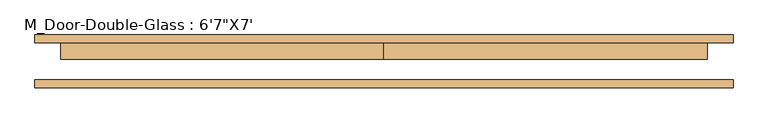
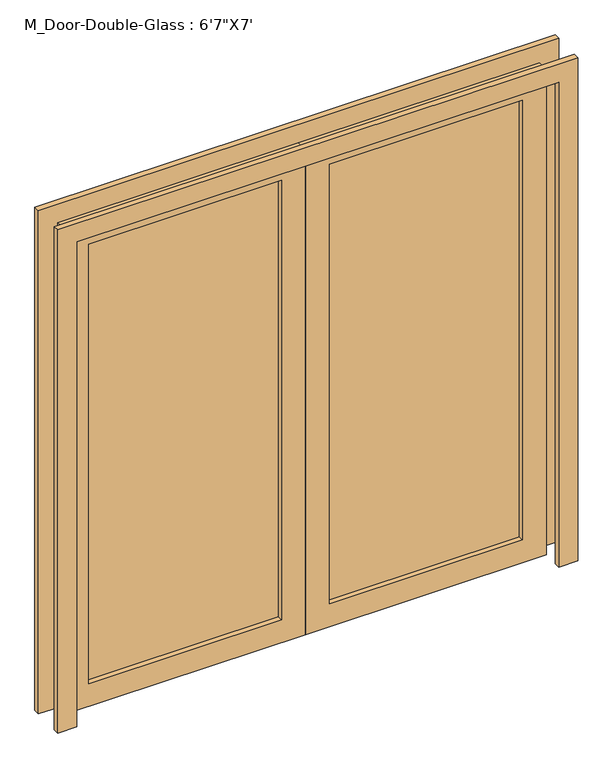
"""IFC4 building model written with IfcOpenShell, lengths in millimetres: door geometry."""

from ifc_helpers import new_model, si_unit, frame, origin, place, context, project, spatial, polyline, outline, extrude, source, transform, mapped, element, save


def door_04ab2522(model_context):
    return source(origin(), model_context, "Body", "SweptSolid", [
        extrude(outline(polyline([(2133.6, 1003.3), (2133.6, 0.0), (0.0, 0.0), (0.0, 1003.3), (2133.6, 1003.3)]), holes=[polyline([(2033.6, 903.3), (100.0, 903.3), (100.0, 100.0), (2033.6, 100.0), (2033.6, 903.3)])]), frame((0.0, 9.53125, 0.0), z_axis=(0.0, 1.0, 0.0), x_axis=(0.0, 0.0, 1.0)), (0.0, 0.0, 1.0), 50.0),
        extrude(outline(polyline([(2133.6, -1003.3), (0.0, -1003.3), (0.0, 0.0), (2133.6, 0.0), (2133.6, -1003.3)]), holes=[polyline([(2033.6, -903.3), (2033.6, -100.0), (100.0, -100.0), (100.0, -903.3), (2033.6, -903.3)])]), frame((0.0, 9.53125, 0.0), z_axis=(0.0, 1.0, 0.0), x_axis=(0.0, 0.0, 1.0)), (0.0, 0.0, 1.0), 50.0),
        extrude(outline(polyline([(-903.3, 37.70625), (-100.0, 37.70625), (-100.0, 31.35625), (-903.3, 31.35625), (-903.3, 37.70625)])), frame((0.0, 0.0, 100.0), z_axis=(0.0, 0.0, 1.0), x_axis=(1.0, 0.0, 0.0)), (0.0, 0.0, 1.0), 1933.6),
        extrude(outline(polyline([(100.0, 37.70625), (903.3, 37.70625), (903.3, 31.35625), (100.0, 31.35625), (100.0, 37.70625)])), frame((0.0, 0.0, 100.0), z_axis=(0.0, 0.0, 1.0), x_axis=(1.0, 0.0, 0.0)), (0.0, 0.0, 1.0), 1933.6),
        extrude(outline(polyline([(0.0, 1083.3), (2213.6, 1083.3), (2213.6, -1083.3), (0.0, -1083.3), (0.0, -1003.3), (2133.6, -1003.3), (2133.6, 1003.3), (0.0, 1003.3), (0.0, 1083.3)])), frame((0.0, -79.76875, 0.0), z_axis=(0.0, 1.0, 0.0), x_axis=(0.0, 0.0, 1.0)), (0.0, 0.0, 1.0), 25.0),
        extrude(outline(polyline([(0.0, 1083.3), (2213.6, 1083.3), (2213.6, -1083.3), (0.0, -1083.3), (0.0, -1003.3), (2133.6, -1003.3), (2133.6, 1003.3), (0.0, 1003.3), (0.0, 1083.3)])), frame((0.0, 59.53125, 0.0), z_axis=(0.0, 1.0, 0.0), x_axis=(0.0, 0.0, 1.0)), (0.0, 0.0, 1.0), 25.0),
    ])


if __name__ == "__main__":
    model = new_model("IFC4")
    model_context = context("Model", 3, world=origin())
    ifc_project = project(units=[si_unit("LENGTHUNIT", "METRE", prefix="MILLI")], contexts=[model_context])
    site = spatial("IfcSite", under=ifc_project)
    building = spatial("IfcBuilding", under=site)
    placement = place(None, origin())
    door_shape = door_04ab2522(model_context)
    element("IfcDoor", 1, ObjectType="M_Door-Double-Glass : 6'7\"X7'", at=placement, inside=building, context=model_context, shape_type="MappedRepresentation", body=[
        mapped(door_shape, transform((0.0, 0.0, 0.0), x_axis=(1.0, 0.0, 0.0), y_axis=(0.0, 1.0, 0.0), z_axis=(0.0, 0.0, 1.0))),
    ])
    save(model, "model.ifc")

# Revit data of these elements
# Type "M_Door-Double-Glass : 6'7\"X7'"
#   Type Mark = "16"
#   Construction Type Id = "opn-d45"
#   Assembly Code = "C1020"
#   Analytic Construction = "Wood frame, double glass door "
#   W = 3' - 3 1/2"
#   Thickness = 0' - 1.9685"
#   Thermal Resistance (R) = 1.8150 (h·ft²·°F)/BTU
#   Swing Angle [instance default] = 90.00°
#   Heat Transfer Coefficient (U) = 0.5510 BTU/(h·ft²·°F)
#   Height = 7' - 0"
#   Bottom Rail = 0' - 3.93701"
#   Top Rail = 0' - 3.93701"
#   Stiles = 0' - 3.93701"
#   Trim Projection = 0' - 0.98425"
#   Trim Width = 0' - 3.14961"
#   Width = 6' - 7"
#   Define Thermal Properties by = 1
#   Glazing = Glass
#   Panel Material = Wood - Birch - Solid Stained Light Low Gloss
#   Trim Material = Paint - Sienna
#   Visual Light Transmittance = 0
#   Solar Heat Gain Coefficient = 0
#   Function = (empty or 0)
#   Wall Closure = (empty or 0)
# Element 1 (IfcDoor, "M_Door-Double-Glass : 6'7\"X7'")
#   Materials on its faces: "Wood - Birch - Solid Stained Light Low Gloss", "Paint - Sienna", "Glass"
# Materials
#   "Glass": class "Glass", colour RGB 0 128 192, transparency 0.75, Description = "Soda Lime Glass", Cost = 0
#   "Wood - Birch - Solid Stained Light Low Gloss": class "Wood", colour RGB 210 159 95, transparency 0, Cost = 0
#   "Paint - Sienna": colour RGB 118 70 51, transparency 0, Cost = 0
